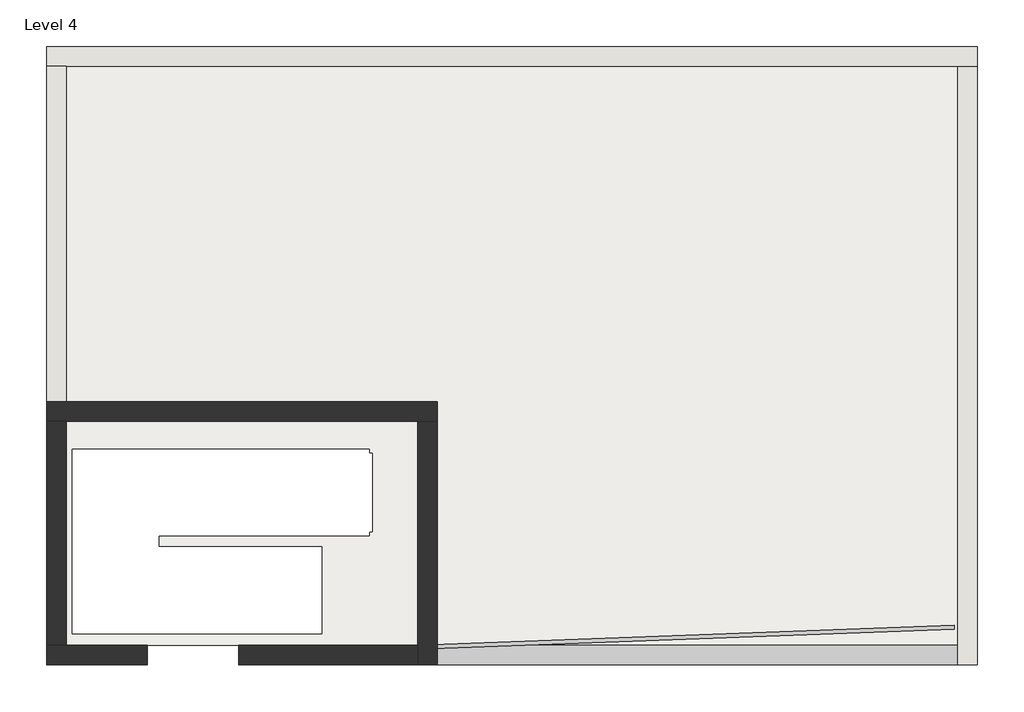
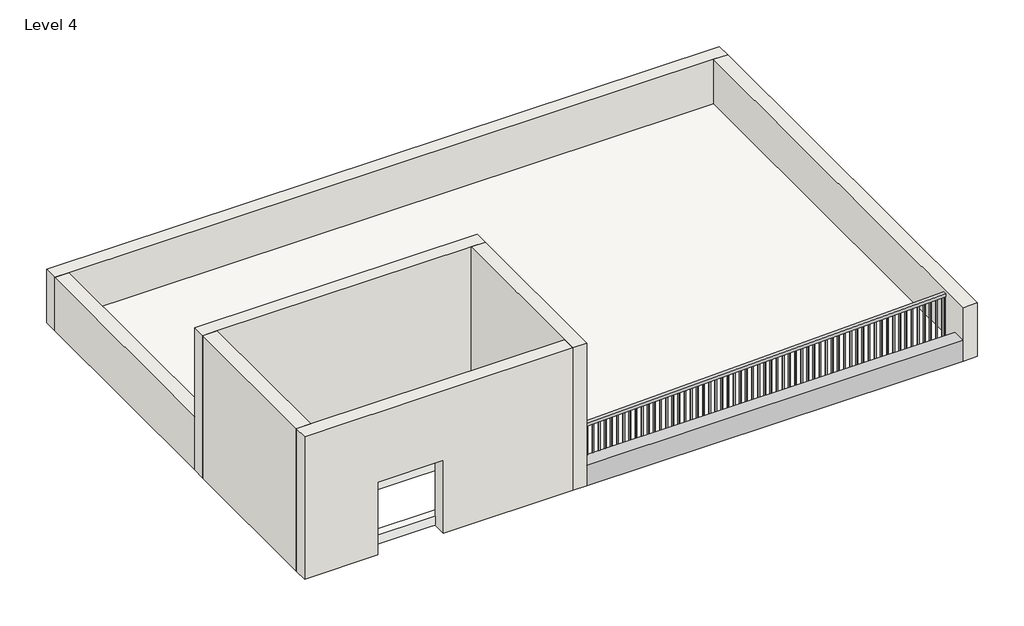
# One storey: 7 walls, 1 proxy, 1 railing, 1 roof.
"""IFC4 building model written with IfcOpenShell, lengths in millimetres."""

from ifc_helpers import new_model, si_unit, frame, origin, place, context, project, spatial, polyline, outline, extrude, faceted_brep, transform, mapped, element, save
from components import generic_models_1_generic_models_1_ce325797

model = new_model("IFC4")

# Units and contexts
model_context = context("Model", 3, world=origin())
ifc_project = project(units=[si_unit("LENGTHUNIT", "METRE", prefix="MILLI")], contexts=[model_context])

# Site, building, storey
site = spatial("IfcSite", under=ifc_project)
building = spatial("IfcBuilding", under=site)
storey = spatial("IfcBuildingStorey", under=building, Name="Level 4", Elevation=6400.8)

# Proxy
placement = place(None, origin())
generic_models_1_generic_models_1_shape = generic_models_1_generic_models_1_ce325797(model_context)
element("IfcBuildingElementProxy", 1, Name="Generic Models 1 : Generic Models 1", ObjectType="Generic Models 1 : Generic Models 1", at=placement, inside=storey, context=model_context, shape_type="MappedRepresentation", body=[
    mapped(generic_models_1_generic_models_1_shape, transform((0.0, 0.0, 0.0), x_axis=(1.0, 0.0, 0.0), y_axis=(0.0, 1.0, 0.0), z_axis=(0.0, 0.0, 1.0))),
])

# Railing
element("IfcRailing", 2, ObjectType="Handrail - Rectangular", at=placement, inside=storey, context=model_context, shape_type="SweptSolid", body=[
    extrude(outline(polyline([(-11342.8807577, -586.2759129), (-11344.774647, -535.5112285), (-5217.2745783, -306.9112285), (-5215.380689, -357.6759129), (-11342.8807577, -586.2759129)])), frame((0.0, 0.0, 7264.4), z_axis=(0.0, 0.0, 1.0), x_axis=(1.0, 0.0, 0.0)), (0.0, 0.0, 1.0), 50.8),
    extrude(outline(polyline([(-5261.2288471, -343.5003365), (-5261.9390556, -324.4635799), (-5242.902299, -323.7533714), (-5242.1920905, -342.790128), (-5261.2288471, -343.5003365)])), frame((0.0, 0.0, 6400.8), z_axis=(0.0, 0.0, 1.0), x_axis=(1.0, 0.0, 0.0)), (0.0, 0.0, 1.0), 863.6),
    extrude(outline(polyline([(-5362.758216, -347.2881151), (-5363.4684245, -328.2513585), (-5344.4316678, -327.54115), (-5343.7214593, -346.5779066), (-5362.758216, -347.2881151)])), frame((0.0, 0.0, 6400.8), z_axis=(0.0, 0.0, 1.0), x_axis=(1.0, 0.0, 0.0)), (0.0, 0.0, 1.0), 863.6),
    extrude(outline(polyline([(-5464.2875848, -351.0758937), (-5464.9977933, -332.0391371), (-5445.9610366, -331.3289286), (-5445.2508281, -350.3656852), (-5464.2875848, -351.0758937)])), frame((0.0, 0.0, 6400.8), z_axis=(0.0, 0.0, 1.0), x_axis=(1.0, 0.0, 0.0)), (0.0, 0.0, 1.0), 863.6),
    extrude(outline(polyline([(-5565.8169536, -354.8636723), (-5566.5271621, -335.8269157), (-5547.4904054, -335.1167072), (-5546.780197, -354.1534639), (-5565.8169536, -354.8636723)])), frame((0.0, 0.0, 6400.8), z_axis=(0.0, 0.0, 1.0), x_axis=(1.0, 0.0, 0.0)), (0.0, 0.0, 1.0), 863.6),
    extrude(outline(polyline([(-5667.3463224, -358.651451), (-5668.0565309, -339.6146943), (-5649.0197743, -338.9044858), (-5648.3095658, -357.9412425), (-5667.3463224, -358.651451)])), frame((0.0, 0.0, 6400.8), z_axis=(0.0, 0.0, 1.0), x_axis=(1.0, 0.0, 0.0)), (0.0, 0.0, 1.0), 863.6),
    extrude(outline(polyline([(-5768.8756912, -362.4392296), (-5769.5858997, -343.4024729), (-5750.5491431, -342.6922644), (-5749.8389346, -361.7290211), (-5768.8756912, -362.4392296)])), frame((0.0, 0.0, 6400.8), z_axis=(0.0, 0.0, 1.0), x_axis=(1.0, 0.0, 0.0)), (0.0, 0.0, 1.0), 863.6),
    extrude(outline(polyline([(-5870.4050601, -366.2270082), (-5871.1152686, -347.1902515), (-5852.0785119, -346.480043), (-5851.3683034, -365.5167997), (-5870.4050601, -366.2270082)])), frame((0.0, 0.0, 6400.8), z_axis=(0.0, 0.0, 1.0), x_axis=(1.0, 0.0, 0.0)), (0.0, 0.0, 1.0), 863.6),
    extrude(outline(polyline([(-5971.9344289, -370.0147868), (-5972.6446374, -350.9780301), (-5953.6078807, -350.2678217), (-5952.8976722, -369.3045783), (-5971.9344289, -370.0147868)])), frame((0.0, 0.0, 6400.8), z_axis=(0.0, 0.0, 1.0), x_axis=(1.0, 0.0, 0.0)), (0.0, 0.0, 1.0), 863.6),
    extrude(outline(polyline([(-6073.4637977, -373.8025654), (-6074.1740062, -354.7658088), (-6055.1372495, -354.0556003), (-6054.4270411, -373.0923569), (-6073.4637977, -373.8025654)])), frame((0.0, 0.0, 6400.8), z_axis=(0.0, 0.0, 1.0), x_axis=(1.0, 0.0, 0.0)), (0.0, 0.0, 1.0), 863.6),
    extrude(outline(polyline([(-6174.9931665, -377.590344), (-6175.703375, -358.5535874), (-6156.6666184, -357.8433789), (-6155.9564099, -376.8801355), (-6174.9931665, -377.590344)])), frame((0.0, 0.0, 6400.8), z_axis=(0.0, 0.0, 1.0), x_axis=(1.0, 0.0, 0.0)), (0.0, 0.0, 1.0), 863.6),
    extrude(outline(polyline([(-6276.5225354, -381.3781226), (-6277.2327438, -362.341366), (-6258.1959872, -361.6311575), (-6257.4857787, -380.6679141), (-6276.5225354, -381.3781226)])), frame((0.0, 0.0, 6400.8), z_axis=(0.0, 0.0, 1.0), x_axis=(1.0, 0.0, 0.0)), (0.0, 0.0, 1.0), 863.6),
    extrude(outline(polyline([(-6378.0519042, -385.1659013), (-6378.7621127, -366.1291446), (-6359.725356, -365.4189361), (-6359.0151475, -384.4556928), (-6378.0519042, -385.1659013)])), frame((0.0, 0.0, 6400.8), z_axis=(0.0, 0.0, 1.0), x_axis=(1.0, 0.0, 0.0)), (0.0, 0.0, 1.0), 863.6),
    extrude(outline(polyline([(-6479.581273, -388.9536799), (-6480.2914815, -369.9169232), (-6461.2547248, -369.2067147), (-6460.5445163, -388.2434714), (-6479.581273, -388.9536799)])), frame((0.0, 0.0, 6400.8), z_axis=(0.0, 0.0, 1.0), x_axis=(1.0, 0.0, 0.0)), (0.0, 0.0, 1.0), 863.6),
    extrude(outline(polyline([(-6581.1106418, -392.7414585), (-6581.8208503, -373.7047018), (-6562.7840937, -372.9944933), (-6562.0738852, -392.03125), (-6581.1106418, -392.7414585)])), frame((0.0, 0.0, 6400.8), z_axis=(0.0, 0.0, 1.0), x_axis=(1.0, 0.0, 0.0)), (0.0, 0.0, 1.0), 863.6),
    extrude(outline(polyline([(-6682.6400106, -396.5292371), (-6683.3502191, -377.4924804), (-6664.3134625, -376.7822719), (-6663.603254, -395.8190286), (-6682.6400106, -396.5292371)])), frame((0.0, 0.0, 6400.8), z_axis=(0.0, 0.0, 1.0), x_axis=(1.0, 0.0, 0.0)), (0.0, 0.0, 1.0), 863.6),
    extrude(outline(polyline([(-6784.1693795, -400.3170157), (-6784.8795879, -381.280259), (-6765.8428313, -380.5700506), (-6765.1326228, -399.6068072), (-6784.1693795, -400.3170157)])), frame((0.0, 0.0, 6400.8), z_axis=(0.0, 0.0, 1.0), x_axis=(1.0, 0.0, 0.0)), (0.0, 0.0, 1.0), 863.6),
    extrude(outline(polyline([(-6885.6987483, -404.1047943), (-6886.4089568, -385.0680377), (-6867.3722001, -384.3578292), (-6866.6619916, -403.3945858), (-6885.6987483, -404.1047943)])), frame((0.0, 0.0, 6400.8), z_axis=(0.0, 0.0, 1.0), x_axis=(1.0, 0.0, 0.0)), (0.0, 0.0, 1.0), 863.6),
    extrude(outline(polyline([(-6987.2281171, -407.8925729), (-6987.9383256, -388.8558163), (-6968.9015689, -388.1456078), (-6968.1913604, -407.1823644), (-6987.2281171, -407.8925729)])), frame((0.0, 0.0, 6400.8), z_axis=(0.0, 0.0, 1.0), x_axis=(1.0, 0.0, 0.0)), (0.0, 0.0, 1.0), 863.6),
    extrude(outline(polyline([(-7088.7574859, -411.6803515), (-7089.4676944, -392.6435949), (-7070.4309378, -391.9333864), (-7069.7207293, -410.9701431), (-7088.7574859, -411.6803515)])), frame((0.0, 0.0, 6400.8), z_axis=(0.0, 0.0, 1.0), x_axis=(1.0, 0.0, 0.0)), (0.0, 0.0, 1.0), 863.6),
    extrude(outline(polyline([(-7190.2868547, -415.4681302), (-7190.9970632, -396.4313735), (-7171.9603066, -395.721165), (-7171.2500981, -414.7579217), (-7190.2868547, -415.4681302)])), frame((0.0, 0.0, 6400.8), z_axis=(0.0, 0.0, 1.0), x_axis=(1.0, 0.0, 0.0)), (0.0, 0.0, 1.0), 863.6),
    extrude(outline(polyline([(-7291.8162236, -419.2559088), (-7292.5264321, -400.2191521), (-7273.4896754, -399.5089436), (-7272.7794669, -418.5457003), (-7291.8162236, -419.2559088)])), frame((0.0, 0.0, 6400.8), z_axis=(0.0, 0.0, 1.0), x_axis=(1.0, 0.0, 0.0)), (0.0, 0.0, 1.0), 863.6),
    extrude(outline(polyline([(-7393.3455924, -423.0436874), (-7394.0558009, -404.0069307), (-7375.0190442, -403.2967222), (-7374.3088357, -422.3334789), (-7393.3455924, -423.0436874)])), frame((0.0, 0.0, 6400.8), z_axis=(0.0, 0.0, 1.0), x_axis=(1.0, 0.0, 0.0)), (0.0, 0.0, 1.0), 863.6),
    extrude(outline(polyline([(-7494.8749612, -426.831466), (-7495.5851697, -407.7947093), (-7476.548413, -407.0845009), (-7475.8382046, -426.1212575), (-7494.8749612, -426.831466)])), frame((0.0, 0.0, 6400.8), z_axis=(0.0, 0.0, 1.0), x_axis=(1.0, 0.0, 0.0)), (0.0, 0.0, 1.0), 863.6),
    extrude(outline(polyline([(-7596.40433, -430.6192446), (-7597.1145385, -411.582488), (-7578.0777819, -410.8722795), (-7577.3675734, -429.9090361), (-7596.40433, -430.6192446)])), frame((0.0, 0.0, 6400.8), z_axis=(0.0, 0.0, 1.0), x_axis=(1.0, 0.0, 0.0)), (0.0, 0.0, 1.0), 863.6),
    extrude(outline(polyline([(-7697.9336988, -434.4070232), (-7698.6439073, -415.3702666), (-7679.6071507, -414.6600581), (-7678.8969422, -433.6968147), (-7697.9336988, -434.4070232)])), frame((0.0, 0.0, 6400.8), z_axis=(0.0, 0.0, 1.0), x_axis=(1.0, 0.0, 0.0)), (0.0, 0.0, 1.0), 863.6),
    extrude(outline(polyline([(-7799.4630677, -438.1948018), (-7800.1732762, -419.1580452), (-7781.1365195, -418.4478367), (-7780.426311, -437.4845933), (-7799.4630677, -438.1948018)])), frame((0.0, 0.0, 6400.8), z_axis=(0.0, 0.0, 1.0), x_axis=(1.0, 0.0, 0.0)), (0.0, 0.0, 1.0), 863.6),
    extrude(outline(polyline([(-7900.9924365, -441.9825804), (-7901.702645, -422.9458238), (-7882.6658883, -422.2356153), (-7881.9556798, -441.272372), (-7900.9924365, -441.9825804)])), frame((0.0, 0.0, 6400.8), z_axis=(0.0, 0.0, 1.0), x_axis=(1.0, 0.0, 0.0)), (0.0, 0.0, 1.0), 863.6),
    extrude(outline(polyline([(-8002.5218053, -445.7703591), (-8003.2320138, -426.7336024), (-7984.1952571, -426.0233939), (-7983.4850487, -445.0601506), (-8002.5218053, -445.7703591)])), frame((0.0, 0.0, 6400.8), z_axis=(0.0, 0.0, 1.0), x_axis=(1.0, 0.0, 0.0)), (0.0, 0.0, 1.0), 863.6),
    extrude(outline(polyline([(-8104.0511741, -449.5581377), (-8104.7613826, -430.521381), (-8085.724626, -429.8111725), (-8085.0144175, -448.8479292), (-8104.0511741, -449.5581377)])), frame((0.0, 0.0, 6400.8), z_axis=(0.0, 0.0, 1.0), x_axis=(1.0, 0.0, 0.0)), (0.0, 0.0, 1.0), 863.6),
    extrude(outline(polyline([(-8205.580543, -453.3459163), (-8206.2907514, -434.3091596), (-8187.2539948, -433.5989511), (-8186.5437863, -452.6357078), (-8205.580543, -453.3459163)])), frame((0.0, 0.0, 6400.8), z_axis=(0.0, 0.0, 1.0), x_axis=(1.0, 0.0, 0.0)), (0.0, 0.0, 1.0), 863.6),
    extrude(outline(polyline([(-8307.1099118, -457.1336949), (-8307.8201203, -438.0969382), (-8288.7833636, -437.3867298), (-8288.0731551, -456.4234864), (-8307.1099118, -457.1336949)])), frame((0.0, 0.0, 6400.8), z_axis=(0.0, 0.0, 1.0), x_axis=(1.0, 0.0, 0.0)), (0.0, 0.0, 1.0), 863.6),
    extrude(outline(polyline([(-8408.6392806, -460.9214735), (-8409.3494891, -441.8847169), (-8390.3127324, -441.1745084), (-8389.6025239, -460.211265), (-8408.6392806, -460.9214735)])), frame((0.0, 0.0, 6400.8), z_axis=(0.0, 0.0, 1.0), x_axis=(1.0, 0.0, 0.0)), (0.0, 0.0, 1.0), 863.6),
    extrude(outline(polyline([(-8510.1686494, -464.7092521), (-8510.8788579, -445.6724955), (-8491.8421012, -444.962287), (-8491.1318928, -463.9990436), (-8510.1686494, -464.7092521)])), frame((0.0, 0.0, 6400.8), z_axis=(0.0, 0.0, 1.0), x_axis=(1.0, 0.0, 0.0)), (0.0, 0.0, 1.0), 863.6),
    extrude(outline(polyline([(-8611.6980182, -468.4970307), (-8612.4082267, -449.4602741), (-8593.3714701, -448.7500656), (-8592.6612616, -467.7868223), (-8611.6980182, -468.4970307)])), frame((0.0, 0.0, 6400.8), z_axis=(0.0, 0.0, 1.0), x_axis=(1.0, 0.0, 0.0)), (0.0, 0.0, 1.0), 863.6),
    extrude(outline(polyline([(-8713.2273871, -472.2848094), (-8713.9375955, -453.2480527), (-8694.9008389, -452.5378442), (-8694.1906304, -471.5746009), (-8713.2273871, -472.2848094)])), frame((0.0, 0.0, 6400.8), z_axis=(0.0, 0.0, 1.0), x_axis=(1.0, 0.0, 0.0)), (0.0, 0.0, 1.0), 863.6),
    extrude(outline(polyline([(-8814.7567559, -476.072588), (-8815.4669644, -457.0358313), (-8796.4302077, -456.3256228), (-8795.7199992, -475.3623795), (-8814.7567559, -476.072588)])), frame((0.0, 0.0, 6400.8), z_axis=(0.0, 0.0, 1.0), x_axis=(1.0, 0.0, 0.0)), (0.0, 0.0, 1.0), 863.6),
    extrude(outline(polyline([(-8916.2861247, -479.8603666), (-8916.9963332, -460.8236099), (-8897.9595765, -460.1134014), (-8897.249368, -479.1501581), (-8916.2861247, -479.8603666)])), frame((0.0, 0.0, 6400.8), z_axis=(0.0, 0.0, 1.0), x_axis=(1.0, 0.0, 0.0)), (0.0, 0.0, 1.0), 863.6),
    extrude(outline(polyline([(-9017.8154935, -483.6481452), (-9018.525702, -464.6113885), (-8999.4889454, -463.90118), (-8998.7787369, -482.9379367), (-9017.8154935, -483.6481452)])), frame((0.0, 0.0, 6400.8), z_axis=(0.0, 0.0, 1.0), x_axis=(1.0, 0.0, 0.0)), (0.0, 0.0, 1.0), 863.6),
    extrude(outline(polyline([(-9119.3448623, -487.4359238), (-9120.0550708, -468.3991672), (-9101.0183142, -467.6889587), (-9100.3081057, -486.7257153), (-9119.3448623, -487.4359238)])), frame((0.0, 0.0, 6400.8), z_axis=(0.0, 0.0, 1.0), x_axis=(1.0, 0.0, 0.0)), (0.0, 0.0, 1.0), 863.6),
    extrude(outline(polyline([(-9220.8742312, -491.2237024), (-9221.5844397, -472.1869458), (-9202.547683, -471.4767373), (-9201.8374745, -490.5134939), (-9220.8742312, -491.2237024)])), frame((0.0, 0.0, 6400.8), z_axis=(0.0, 0.0, 1.0), x_axis=(1.0, 0.0, 0.0)), (0.0, 0.0, 1.0), 863.6),
    extrude(outline(polyline([(-9322.4036, -495.011481), (-9323.1138085, -475.9747244), (-9304.0770518, -475.2645159), (-9303.3668433, -494.3012725), (-9322.4036, -495.011481)])), frame((0.0, 0.0, 6400.8), z_axis=(0.0, 0.0, 1.0), x_axis=(1.0, 0.0, 0.0)), (0.0, 0.0, 1.0), 863.6),
    extrude(outline(polyline([(-9423.9329688, -498.7992596), (-9424.6431773, -479.762503), (-9405.6064206, -479.0522945), (-9404.8962121, -498.0890512), (-9423.9329688, -498.7992596)])), frame((0.0, 0.0, 6400.8), z_axis=(0.0, 0.0, 1.0), x_axis=(1.0, 0.0, 0.0)), (0.0, 0.0, 1.0), 863.6),
    extrude(outline(polyline([(-9525.4623376, -502.5870383), (-9526.1725461, -483.5502816), (-9507.1357895, -482.8400731), (-9506.425581, -501.8768298), (-9525.4623376, -502.5870383)])), frame((0.0, 0.0, 6400.8), z_axis=(0.0, 0.0, 1.0), x_axis=(1.0, 0.0, 0.0)), (0.0, 0.0, 1.0), 863.6),
    extrude(outline(polyline([(-9626.9917064, -506.3748169), (-9627.7019149, -487.3380602), (-9608.6651583, -486.6278517), (-9607.9549498, -505.6646084), (-9626.9917064, -506.3748169)])), frame((0.0, 0.0, 6400.8), z_axis=(0.0, 0.0, 1.0), x_axis=(1.0, 0.0, 0.0)), (0.0, 0.0, 1.0), 863.6),
    extrude(outline(polyline([(-9728.5210753, -510.1625955), (-9729.2312838, -491.1258388), (-9710.1945271, -490.4156303), (-9709.4843186, -509.452387), (-9728.5210753, -510.1625955)])), frame((0.0, 0.0, 6400.8), z_axis=(0.0, 0.0, 1.0), x_axis=(1.0, 0.0, 0.0)), (0.0, 0.0, 1.0), 863.6),
    extrude(outline(polyline([(-9830.0504441, -513.9503741), (-9830.7606526, -494.9136174), (-9811.7238959, -494.203409), (-9811.0136874, -513.2401656), (-9830.0504441, -513.9503741)])), frame((0.0, 0.0, 6400.8), z_axis=(0.0, 0.0, 1.0), x_axis=(1.0, 0.0, 0.0)), (0.0, 0.0, 1.0), 863.6),
    extrude(outline(polyline([(-9931.5798129, -517.7381527), (-9932.2900214, -498.7013961), (-9913.2532647, -497.9911876), (-9912.5430563, -517.0279442), (-9931.5798129, -517.7381527)])), frame((0.0, 0.0, 6400.8), z_axis=(0.0, 0.0, 1.0), x_axis=(1.0, 0.0, 0.0)), (0.0, 0.0, 1.0), 863.6),
    extrude(outline(polyline([(-10033.1091817, -521.5259313), (-10033.8193902, -502.4891747), (-10014.7826336, -501.7789662), (-10014.0724251, -520.8157228), (-10033.1091817, -521.5259313)])), frame((0.0, 0.0, 6400.8), z_axis=(0.0, 0.0, 1.0), x_axis=(1.0, 0.0, 0.0)), (0.0, 0.0, 1.0), 863.6),
    extrude(outline(polyline([(-10134.6385505, -525.3137099), (-10135.348759, -506.2769533), (-10116.3120024, -505.5667448), (-10115.6017939, -524.6035014), (-10134.6385505, -525.3137099)])), frame((0.0, 0.0, 6400.8), z_axis=(0.0, 0.0, 1.0), x_axis=(1.0, 0.0, 0.0)), (0.0, 0.0, 1.0), 863.6),
    extrude(outline(polyline([(-10236.1679194, -529.1014886), (-10236.8781279, -510.0647319), (-10217.8413712, -509.3545234), (-10217.1311627, -528.3912801), (-10236.1679194, -529.1014886)])), frame((0.0, 0.0, 6400.8), z_axis=(0.0, 0.0, 1.0), x_axis=(1.0, 0.0, 0.0)), (0.0, 0.0, 1.0), 863.6),
    extrude(outline(polyline([(-10337.6972882, -532.8892672), (-10338.4074967, -513.8525105), (-10319.37074, -513.142302), (-10318.6605315, -532.1790587), (-10337.6972882, -532.8892672)])), frame((0.0, 0.0, 6400.8), z_axis=(0.0, 0.0, 1.0), x_axis=(1.0, 0.0, 0.0)), (0.0, 0.0, 1.0), 863.6),
    extrude(outline(polyline([(-10439.226657, -536.6770458), (-10439.9368655, -517.6402891), (-10420.9001088, -516.9300806), (-10420.1899004, -535.9668373), (-10439.226657, -536.6770458)])), frame((0.0, 0.0, 6400.8), z_axis=(0.0, 0.0, 1.0), x_axis=(1.0, 0.0, 0.0)), (0.0, 0.0, 1.0), 863.6),
    extrude(outline(polyline([(-10540.7560258, -540.4648244), (-10541.4662343, -521.4280677), (-10522.4294777, -520.7178592), (-10521.7192692, -539.7546159), (-10540.7560258, -540.4648244)])), frame((0.0, 0.0, 6400.8), z_axis=(0.0, 0.0, 1.0), x_axis=(1.0, 0.0, 0.0)), (0.0, 0.0, 1.0), 863.6),
    extrude(outline(polyline([(-10642.2853947, -544.252603), (-10642.9956031, -525.2158464), (-10623.9588465, -524.5056379), (-10623.248638, -543.5423945), (-10642.2853947, -544.252603)])), frame((0.0, 0.0, 6400.8), z_axis=(0.0, 0.0, 1.0), x_axis=(1.0, 0.0, 0.0)), (0.0, 0.0, 1.0), 863.6),
    extrude(outline(polyline([(-10743.8147635, -548.0403816), (-10744.524972, -529.003625), (-10725.4882153, -528.2934165), (-10724.7780068, -547.3301731), (-10743.8147635, -548.0403816)])), frame((0.0, 0.0, 6400.8), z_axis=(0.0, 0.0, 1.0), x_axis=(1.0, 0.0, 0.0)), (0.0, 0.0, 1.0), 863.6),
    extrude(outline(polyline([(-10845.3441323, -551.8281602), (-10846.0543408, -532.7914036), (-10827.0175841, -532.0811951), (-10826.3073756, -551.1179517), (-10845.3441323, -551.8281602)])), frame((0.0, 0.0, 6400.8), z_axis=(0.0, 0.0, 1.0), x_axis=(1.0, 0.0, 0.0)), (0.0, 0.0, 1.0), 863.6),
    extrude(outline(polyline([(-10946.8735011, -555.6159388), (-10947.5837096, -536.5791822), (-10928.546953, -535.8689737), (-10927.8367445, -554.9057304), (-10946.8735011, -555.6159388)])), frame((0.0, 0.0, 6400.8), z_axis=(0.0, 0.0, 1.0), x_axis=(1.0, 0.0, 0.0)), (0.0, 0.0, 1.0), 863.6),
    extrude(outline(polyline([(-11048.4028699, -559.4037175), (-11049.1130784, -540.3669608), (-11030.0763218, -539.6567523), (-11029.3661133, -558.693509), (-11048.4028699, -559.4037175)])), frame((0.0, 0.0, 6400.8), z_axis=(0.0, 0.0, 1.0), x_axis=(1.0, 0.0, 0.0)), (0.0, 0.0, 1.0), 863.6),
    extrude(outline(polyline([(-11149.9322388, -563.1914961), (-11150.6424472, -544.1547394), (-11131.6056906, -543.4445309), (-11130.8954821, -562.4812876), (-11149.9322388, -563.1914961)])), frame((0.0, 0.0, 6400.8), z_axis=(0.0, 0.0, 1.0), x_axis=(1.0, 0.0, 0.0)), (0.0, 0.0, 1.0), 863.6),
    extrude(outline(polyline([(-11251.4616076, -566.9792747), (-11252.1718161, -547.942518), (-11233.1350594, -547.2323095), (-11232.4248509, -566.2690662), (-11251.4616076, -566.9792747)])), frame((0.0, 0.0, 6400.8), z_axis=(0.0, 0.0, 1.0), x_axis=(1.0, 0.0, 0.0)), (0.0, 0.0, 1.0), 863.6),
    extrude(outline(polyline([(-5235.009286, -342.5221575), (-5235.7194945, -323.4854009), (-5216.6827379, -322.7751924), (-5215.9725294, -341.8119491), (-5235.009286, -342.5221575)])), frame((0.0, 0.0, 6400.8), z_axis=(0.0, 0.0, 1.0), x_axis=(1.0, 0.0, 0.0)), (0.0, 0.0, 1.0), 863.6),
    extrude(outline(polyline([(-11343.4725981, -570.4119491), (-11344.1828066, -551.3751924), (-11325.1460499, -550.6649839), (-11324.4358414, -569.7017406), (-11343.4725981, -570.4119491)])), frame((0.0, 0.0, 6400.8), z_axis=(0.0, 0.0, 1.0), x_axis=(1.0, 0.0, 0.0)), (0.0, 0.0, 1.0), 863.6),
])

# Roof
element("IfcRoof", 3, ObjectType="ROOFING 6\"", at=placement, inside=storey, context=model_context, shape_type="SweptSolid", body=[
    extrude(outline(polyline([(-15611.0277023, 6236.3679075), (-5171.6277023, 6236.3679075), (-5171.6277023, -545.4320925), (-15611.0277023, -545.4320925), (-15611.0277023, 6236.3679075)]), holes=[polyline([(-12061.3777023, 788.0679075), (-12029.6277023, 788.0679075), (-12029.6277023, 1702.4679075), (-12061.3777023, 1702.4679075), (-12061.3777023, 1753.2679075), (-15541.1777023, 1753.2679075), (-15541.1777023, -405.7320925), (-12620.1777023, -405.7320925), (-12620.1777023, 610.2679075), (-14525.1777023, 610.2679075), (-14525.1777023, 737.2679075), (-12061.3777023, 737.2679075), (-12061.3777023, 788.0679075)])]), frame((0.0, 0.0, 6400.8), z_axis=(0.0, 0.0, 1.0), x_axis=(1.0, 0.0, 0.0)), (0.0, 0.0, 1.0), 152.4),
])

# Walls
element("IfcWall", 4, ObjectType="OUTER Wall 9\"", at=placement, inside=storey, context=model_context, shape_type="Brep", body=[
    faceted_brep([(-15839.6277023, 6236.3679075, 6400.8), (-15611.0277023, 6236.3679075, 6400.8), (-5171.6277023, 6236.3679075, 6400.8), (-4943.0277023, 6236.3679075, 6400.8), (-4943.0277023, 6236.3679075, 7315.2), (-5171.6277023, 6236.3679075, 7315.2), (-15611.0277023, 6236.3679075, 7315.2), (-15839.6277023, 6236.3679075, 7315.2), (-15839.6277023, 6464.9679075, 6400.8), (-15839.6277023, 6464.9679075, 7315.2), (-4943.0277023, 6464.9679075, 7315.2), (-4943.0277023, 6464.9679075, 6400.8)], [[[0, 1, 2, 3, 4, 5, 6, 7]], [[8, 9, 10, 11]], [[3, 2, 1, 0, 8, 11]], [[7, 6, 5, 4, 10, 9]], [[4, 3, 11, 10]], [[0, 7, 9, 8]]]),
])
element("IfcWall", 5, ObjectType="OUTER Wall 9\"", at=placement, inside=storey, context=model_context, shape_type="SweptSolid", body=[
    extrude(outline(polyline([(-5171.6277023, -774.0320925), (-5171.6277023, 6236.3679075), (-4943.0277023, 6236.3679075), (-4943.0277023, -774.0320925), (-5171.6277023, -774.0320925)])), frame((0.0, 0.0, 6400.8), z_axis=(0.0, 0.0, 1.0), x_axis=(1.0, 0.0, 0.0)), (0.0, 0.0, 1.0), 914.4),
])
element("IfcWall", 6, ObjectType="OUTER Wall 9\"", at=placement, inside=storey, context=model_context, shape_type="Brep", body=[
    faceted_brep([(-15839.6277023, 2080.7064293, 8839.2), (-15839.6277023, 2080.7064293, 6400.8), (-15611.0277023, 2080.7064293, 6400.8), (-11496.2277023, 2080.7064293, 6400.8), (-11267.6277023, 2080.7064293, 6400.8), (-11267.6277023, 2080.7064293, 8839.2), (-11496.2277023, 2080.7064293, 8839.2), (-15611.0277023, 2080.7064293, 8839.2), (-15839.6277023, 2309.3064293, 6400.8), (-15839.6277023, 2309.3064293, 7315.2), (-15839.6277023, 2309.3064293, 8839.2), (-11267.6277023, 2309.3064293, 8839.2), (-11267.6277023, 2309.3064293, 6400.8), (-15611.0277023, 2309.3064293, 6400.8)], [[[0, 1, 2, 3, 4, 5, 6, 7]], [[8, 9, 10, 11, 12, 13]], [[4, 3, 2, 1, 8, 13, 12]], [[0, 7, 6, 5, 11, 10]], [[5, 4, 12, 11]], [[0, 10, 9, 8, 1]]]),
])
element("IfcWall", 7, ObjectType="OUTER Wall 9\"", at=placement, inside=storey, context=model_context, shape_type="Brep", body=[
    faceted_brep([(-11496.2277023, 2080.7064293, 6400.8), (-11496.2277023, -545.4320925, 6400.8), (-11496.2277023, -774.0320925, 6400.8), (-11496.2277023, -774.0320925, 8839.2), (-11496.2277023, -545.4320925, 8839.2), (-11496.2277023, 2080.7064293, 8839.2), (-11267.6277023, 2080.7064293, 6400.8), (-11267.6277023, 2080.7064293, 8839.2), (-11267.6277023, -774.0320925, 8839.2), (-11267.6277023, -774.0320925, 6400.8)], [[[0, 1, 2, 3, 4, 5]], [[6, 7, 8, 9]], [[2, 1, 0, 6, 9]], [[5, 4, 3, 8, 7]], [[0, 5, 7, 6]], [[3, 2, 9, 8]]]),
])
element("IfcWall", 8, ObjectType="OUTER Wall 9\"", at=placement, inside=storey, context=model_context, shape_type="Brep", body=[
    faceted_brep([(-15839.6277023, -545.4320925, 8839.2), (-15611.0277023, -545.4320925, 8839.2), (-11496.2277023, -545.4320925, 8839.2), (-11496.2277023, -545.4320925, 6400.8), (-13591.7277023, -545.4320925, 6400.8), (-13591.7277023, -545.4320925, 7647.3395593), (-14658.5277023, -545.4320925, 7647.3395593), (-14658.5277023, -545.4320925, 6400.8), (-15611.0277023, -545.4320925, 6400.8), (-15839.6277023, -545.4320925, 6400.8), (-11496.2277023, -774.0320925, 8839.2), (-15839.6277023, -774.0320925, 8839.2), (-15839.6277023, -774.0320925, 6400.8), (-14658.5277023, -774.0320925, 6400.8), (-14658.5277023, -774.0320925, 7647.3395593), (-13591.7277023, -774.0320925, 7647.3395593), (-13591.7277023, -774.0320925, 6400.8), (-11496.2277023, -774.0320925, 6400.8)], [[[0, 1, 2, 3, 4, 5, 6, 7, 8, 9]], [[10, 11, 12, 13, 14, 15, 16, 17]], [[3, 17, 16, 4]], [[12, 9, 8, 7, 13]], [[2, 1, 0, 11, 10]], [[3, 2, 10, 17]], [[0, 9, 12, 11]], [[6, 14, 13, 7]], [[14, 6, 5, 15]], [[15, 5, 4, 16]]]),
])
element("IfcWall", 9, ObjectType="OUTER Wall 9\"", at=placement, inside=storey, context=model_context, shape_type="SweptSolid", body=[
    extrude(outline(polyline([(-15839.6277023, -545.4320925), (-15839.6277023, 2080.7064293), (-15611.0277023, 2080.7064293), (-15611.0277023, -545.4320925), (-15839.6277023, -545.4320925)])), frame((0.0, 0.0, 6400.8), z_axis=(0.0, 0.0, 1.0), x_axis=(1.0, 0.0, 0.0)), (0.0, 0.0, 1.0), 2438.4),
])
element("IfcWall", 10, ObjectType="OUTER Wall 9\"", at=placement, inside=storey, context=model_context, shape_type="SweptSolid", body=[
    extrude(outline(polyline([(-15839.6277023, 2309.3064293), (-15839.6277023, 6236.3679075), (-15611.0277023, 6236.3679075), (-15611.0277023, 2309.3064293), (-15839.6277023, 2309.3064293)])), frame((0.0, 0.0, 6400.8), z_axis=(0.0, 0.0, 1.0), x_axis=(1.0, 0.0, 0.0)), (0.0, 0.0, 1.0), 914.4),
])

save(model, "model.ifc")

# Revit data of these elements
# Type "Handrail - Rectangular"
#   Assembly Code = "C2010400"
#   built-in parameter 1008612 = 0.0416667 (stored number, unit not read)
#   built-in parameter 1008611 = 0.0416667 (stored number, unit not read)
#   built-in parameter 1008609 = 0.333333 (stored number, unit not read)
#   built-in parameter 1008604 = 0.166667 (stored number, unit not read)
#   built-in parameter 1008603 = 0.166667 (stored number, unit not read)
#   Railing Height = 3' - 0"
#   built-in parameter 1008630 = 2
#   built-in parameter 1008610 = 2
#   built-in parameter 1008618 = Baluster - Square : 3/4"
# Type "ROOFING 6\""
#   Assembly Code = "B1020"
#   Layers, outside or top first: 0' - 6" "ROOFING MATERIAL 6\"" (function 1)
# Type "OUTER Wall 9\""
#   Assembly Code = "B2010"
#   Layers, outside or top first: 0' - 9" "outer wall" (function 1)
# Element 1 (IfcBuildingElementProxy, "Generic Models 1 : Generic Models 1")
#   Phase Created = New Construction
#   Materials on its faces: "Clad - White"
# Element 2 (IfcRailing, "Handrail - Rectangular")
#   Phase Created = New Construction
# Element 3 (IfcRoof, "ROOFING 6\"")
#   built-in parameter 1001705 = 21.5 (stored number, unit not read)
#   built-in parameter 1001710 = 33615
#   Phase Created = New Construction
#   Materials on its faces: "ROOFING MATERIAL 6\""
# Elements 4, 5, 10 (IfcWall, "OUTER Wall 9\"")
#   Top Offset = 0' - 0"
#   Base Offset = 0' - 0"
#   Unconnected Height = 3' - 0"
#   wall height = 3' - 0"
#   Phase Created = New Construction
#   Base Constraint = Level 4
#   Materials on its faces: "outer wall"
# Elements 6, 7, 8, 9 (IfcWall, "OUTER Wall 9\"")
#   Top Offset = 0' - 0"
#   Base Offset = 0' - 0"
#   Unconnected Height = 8' - 0"
#   wall height = 8' - 0"
#   Phase Created = New Construction
#   Base Constraint = Level 4
#   Materials on its faces: "outer wall"
# Materials
#   "ROOFING MATERIAL 6\"": class "Generic", colour RGB 120 120 120, transparency 0, Cost = 0
#   "outer wall": class "Generic", colour RGB 120 120 120, transparency 0, Cost = 0
#   "Clad - White": class "Wood", colour RGB 242 242 238, transparency 0, Cost = 0
